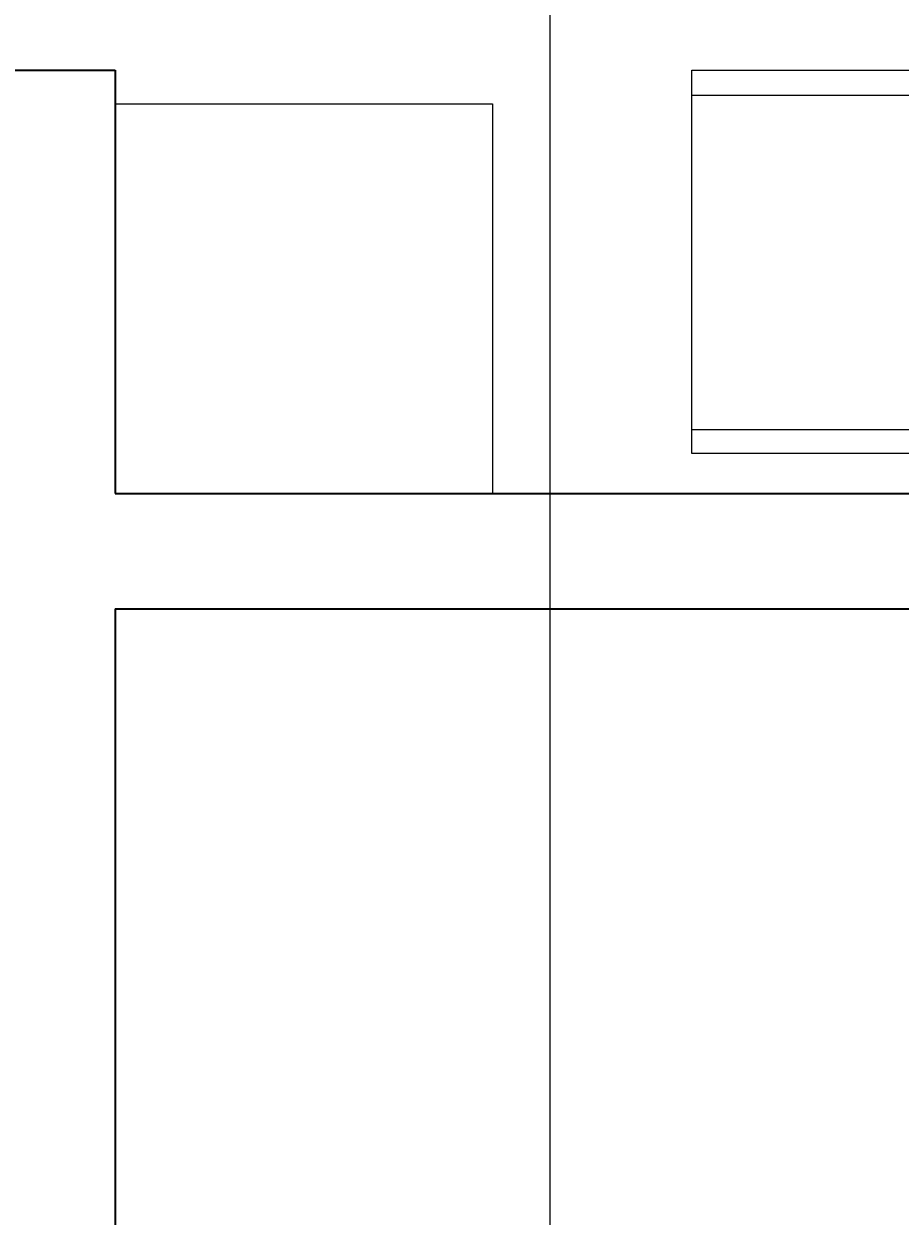
# Model space of a CAD drawing. Units: inches. Extents: x -61 to 1599, y -1316 to 257.
# Tile 90 of 204: x 321 to 367, y -342 to -280. Entities that reach past the tile are written whole.
import ezdxf

# ---------------------------------------------------------------- set-up
doc = ezdxf.new("R2010")
doc.units = ezdxf.units.IN
doc.header["$MEASUREMENT"] = 0
for name, color, linetype, lineweight in [('A-ANNO-DIMS', 2, 'Continuous', 18), ('A-FLOR-CASE', 8, 'Continuous', 18), ('WALLS', 4, 'Continuous', 35)]:
    doc.layers.add(name, color=color, linetype=linetype, lineweight=lineweight)
doc.styles.get("Standard").update_dxf_attribs({"font": 'arial.ttf'})
doc.dimstyles.get("Standard").update_dxf_attribs({"dimtxt": 0.18, "dimasz": 0.18, "dimexe": 0.18, "dimexo": 0.0625, "dimgap": 0.09, "dimtad": 0, "dimtih": 1, "dimtoh": 1, "dimdec": 0, "dimzin": 0, "dimdsep": 46, "dimlunit": 3, "dimtxsty": 'Standard', "dimcen": 0.09, "dimadec": 0, "dimazin": 0, "dimtfac": 1, "dimtdec": 0, "dimtofl": 0, "dimtmove": 0, "dimatfit": 3, "dimfxl": 1, "dimtolj": 1, "dimtzin": 0, "dimarcsym": 0})

# ---------------------------------------------------------------- blocks, each defined once
blk = doc.blocks.new('KITCHEN-BASE-UNIT')
for p, q in [((25.074, 18.599), (0, 18.599)), ((25.074, 1.234), (0, 1.234))]:
    blk.add_line(p, q)
blk.add_lwpolyline([(25.074, 0), (0, 0), (0, 19.922), (25.074, 19.922)], close=True)
blk = doc.blocks.new('*D699')
at = {"layer": 'A-ANNO-DIMS', "color": 0, "lineweight": -2, "transparency": 16777216}
for p, q in [((835.64, -167.169), (-61.077, -167.169)), ((-60.897, -167.349), (-60.897, -306.726)), ((-60.897, -446.466), (-60.897, -307.09)), ((841.64, -446.646), (-61.077, -446.646))]:
    blk.add_line(p, q, dxfattribs=at)
at = {"layer": 'A-ANNO-DIMS', "color": 0, "transparency": 16777216}
for points in [[(-60.927, -167.349), (-60.867, -167.349), (-60.897, -167.169)], [(-60.927, -446.466), (-60.867, -446.466), (-60.897, -446.646)]]:
    blk.add_solid(points, dxfattribs=at)
at = {"layer": 'DEFPOINTS', "color": 0, "transparency": 16777216}
for p in [(835.703, -167.169), (-60.897, -446.646), (841.703, -446.646)]:
    blk.add_point(p, dxfattribs=at)
at = {"layer": 'A-ANNO-DIMS', "color": 0, "transparency": 16777216, "insert": (-60.897, -306.908), "char_height": 0.18, "attachment_point": 5}
blk.add_mtext('\\A1;279.5', dxfattribs=at)
blk = doc.blocks.new('*D702')
at = {"layer": 'A-ANNO-DIMS', "color": 0, "lineweight": -2, "transparency": 16777216}
for p, q in [((276.882, -616.882), (276.882, 257.457)), ((277.062, 257.277), (312.209, 257.277)), ((348.14, 257.277), (312.994, 257.277)), ((348.32, -616.882), (348.32, 257.457))]:
    blk.add_line(p, q, dxfattribs=at)
at = {"layer": 'A-ANNO-DIMS', "color": 0, "transparency": 16777216}
for points in [[(277.062, 257.307), (277.062, 257.247), (276.882, 257.277)], [(348.14, 257.307), (348.14, 257.247), (348.32, 257.277)]]:
    blk.add_solid(points, dxfattribs=at)
at = {"layer": 'DEFPOINTS', "color": 0, "transparency": 16777216}
for p in [(348.32, 257.277), (276.882, -616.945), (348.32, -616.945)]:
    blk.add_point(p, dxfattribs=at)
at = {"layer": 'A-ANNO-DIMS', "color": 0, "transparency": 16777216, "insert": (312.601, 257.277), "char_height": 0.18, "attachment_point": 5}
blk.add_mtext('\\A1;71.44', dxfattribs=at)

msp = doc.modelspace()

# ---------------------------------------------------------------- linework, layer by layer
at = {"layer": 'A-FLOR-CASE'}
msp.add_lwpolyline([(345.3268, -304.3229), (325.7028, -304.3229), (325.7028, -284.0689), (345.3268, -284.0689)], close=True, dxfattribs=at)
at = {"layer": 'WALLS'}
for p, q in [((317.017, -282.3229), (325.7028, -282.3229)), ((325.7028, -282.3229), (325.7028, -304.3229)), ((325.7028, -304.3229), (403.7028, -304.3229)), ((325.7028, -310.3229), (397.7028, -310.3229)), ((325.7028, -310.3229), (325.7028, -376.2211))]:
    msp.add_line(p, q, dxfattribs=at)

# ---------------------------------------------------------------- block references
at = {"layer": 'A-FLOR-CASE'}
msp.add_blockref('KITCHEN-BASE-UNIT', (355.674, -302.245), dxfattribs=at)

# ---------------------------------------------------------------- dimensions: what is measured, and where the dimension line sits
at = {"layer": 'A-ANNO-DIMS'}
dim = msp.add_linear_dim(base=(348.3201, 257.2771), p1=(276.8825, -616.9446), p2=(348.3201, -616.9446), dimstyle='Standard', override={"dimdec": 2, "dimlfac": 1, "dimrnd": 0, "dimzin": 0, "dimdsep": 46, "dimlunit": 2}, dxfattribs=at)
dim.commit()
dim.dimension.update_dxf_attribs({"geometry": '*D702', "text_midpoint": (312.6013, 257.2771)})
dim = msp.add_linear_dim(base=(-60.8972, -446.6462), p1=(835.7028, -167.169), p2=(841.7028, -446.6462), angle=90, dimstyle='Standard', override={"dimdec": 1, "dimlfac": 1, "dimrnd": 0, "dimzin": 0, "dimdsep": 46, "dimlunit": 2}, dxfattribs=at)
dim.commit()
dim.dimension.update_dxf_attribs({"geometry": '*D699', "text_midpoint": (-60.8972, -306.9076)})

doc.saveas('drawing.dxf')
